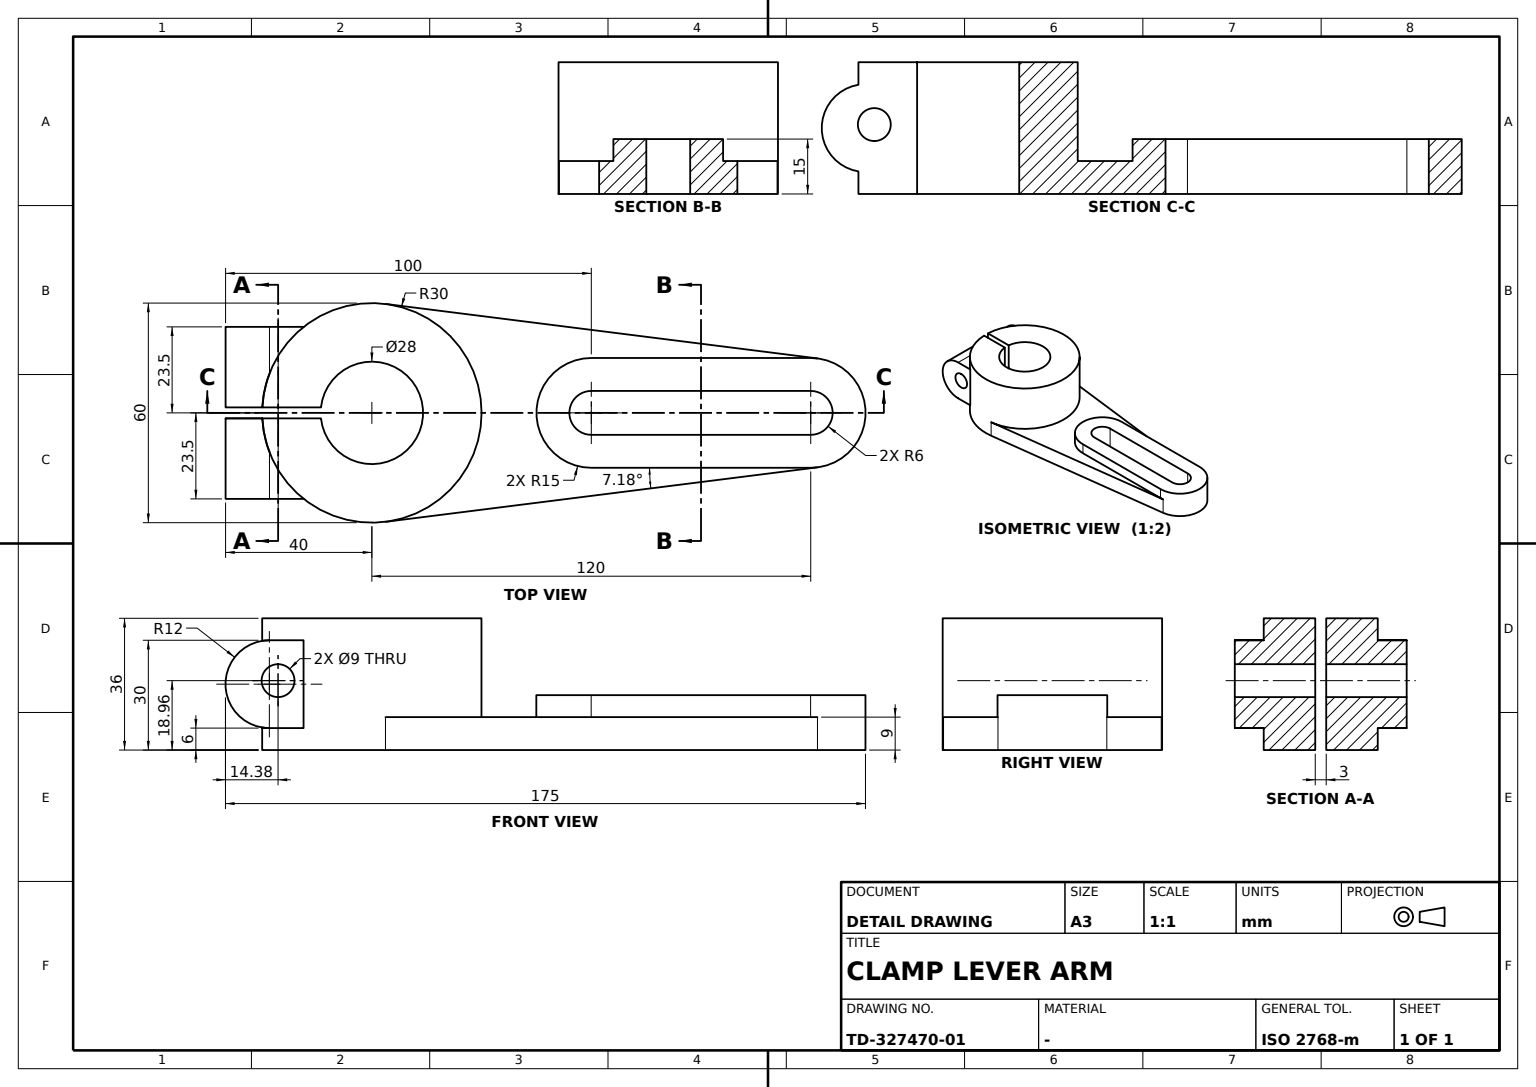
CATIA V5 part; units mm, degrees
sketch "Sketch1" plane through (0, 0, 0) normal (0, 0, 1) x (1, 0, 0)
  circle A0 centre (0, 0) radius 30
  circle A1 centre (0, 0) radius 14
  dimension "radius A1" = 14
  dimension "radius A0" = 30
extrude "Pad1" add sketch "Sketch1" along normal blind 36
sketch "Sketch2" plane through (0, 0, 0) normal (0, 0, 1) x (1, 0, 0)
  line L0 (60, 0) -> (120, 0) construction
  point P0 (60, 0)
  point P1 (120, 0)
  line L1 (60, 15) -> (120, 15)
  line L2 (120, -15) -> (60, -15)
  arc A0 (120, 15) -> (120, -15) centre (120, 0) cw
  arc A1 (60, -15) -> (60, 15) centre (60, 0) cw
  line L3 (60, 0) -> (120, 0) construction
  line L4 (60, 6) -> (120, 6)
  line L5 (120, -6) -> (60, -6)
  arc A2 (120, 6) -> (120, -6) centre (120, 0) cw
  arc A3 (60, -6) -> (60, 6) centre (60, 0) cw
  dimension "distance L0 L1" = 15
  dimension "length L0" = 60
  dimension "distance y axis P1" = 120
  dimension "distance L3 L4" = 6
  constraint coincidence P0 x-axis
  constraint horizontal L0 x-axis
  constraint horizontal L3 x-axis
  constraint tangency A0 L1
  constraint tangency A1 L1
  constraint tangency A0 L2
  constraint tangency A1 L2
  constraint tangency A2 L4
  constraint tangency A3 L4
  constraint tangency A2 L5
  constraint tangency A3 L5
extrude "Pad2" add sketch "Sketch2" along normal blind 15
ref_plane "Plane1" through (0, 0, 3) normal (0, 0, -1) x (1, 0, 0)
sketch "Sketch4" plane through (0, 0, 0) normal (0, 0, -1) x (1, 0, 0)
  circle A0 centre (0, 0) radius 30 construction
  arc A1 (3.75, -29.7647) -> (3.75, 29.7647) centre (0, 0) ccw
  line L0 (120, -15) -> (60, -15)
  point P0 (120, -15)
  arc A2 (120, -15) -> (120, 15) centre (120, 0) ccw construction
  arc A3 (120, -15) -> (121.875, -14.8824) centre (120, 0) ccw
  arc A4 (121.875, 14.8824) -> (120, 15) centre (120, 0) ccw
  point P1 (120, -15)
  point P2 (120, 15)
  line L1 (60, 15) -> (120, 15)
  point P3 (120, 15)
  arc A5 (60, 15) -> (60, -15) centre (60, 0) ccw
  line L2 (3.75, 29.7647) -> (121.875, 14.8824)
  point P4 (3.75, 29.7647)
  point P5 (121.875, 14.8824)
  line L3 (3.75, -29.7647) -> (121.875, -14.8824)
  point P6 (3.75, -29.7647)
  point P7 (121.875, -14.8824)
  constraint tangency L2 A0
  constraint tangency L2 A2
  constraint tangency L3 A0
  constraint tangency L3 A2
  constraint coincidence A0 P4
  constraint coincidence A2 P5
  constraint coincidence A0 P6
  constraint coincidence A2 P7
  constraint coincidence P0 P1
  constraint coincidence P2 P3
extrude "Pad3" add sketch "Sketch4" against normal blind 9
sketch "Sketch5" plane through (0, 0, 0) normal (0, 1, 0) x (-1, 0, 0)
  point P0 (28, 18)
  arc A0 (28, 6) -> (28, 30) centre (28, 18) ccw
  line L0 (28, 30) -> (0, 30)
  point P1 (0, 30)
  line L1 (28, 6) -> (0, 6)
  point P2 (0, 6)
  line L2 (0, 6) -> (0, 30)
  dimension "radius A0" = 12
  dimension "distance P0 x axis" = 18
  dimension "distance y axis P0" = 28
  constraint coincidence P1 y-axis
  constraint coincidence P2 y-axis
  constraint horizontal L0 x-axis
  constraint tangency L1 A0
  constraint vertical L2 y-axis
extrude "Pad4" add sketch "Sketch5" along normal blind 23.5
mirror "Mirror1" about plane through (0, 0, 0) normal (0, 1, 0) of "Pad4"
sketch "Sketch6" plane through (0, 0, 36) normal (0, 0, 1) x (1, 0, 0)
  circle A0 centre (0, 0) radius 14 construction
  arc A1 (-13.9194, -1.5) -> (-13.9194, 1.5) centre (0, 0) ccw
  line L0 (-13.9194, 1.5) -> (-50, 1.5)
  line L1 (-50, 1.5) -> (-50, -1.5)
  line L2 (-50, -1.5) -> (-13.9194, -1.5)
  point P0 (-13.9194, 1.5)
  point P1 (-13.9194, -1.5)
  dimension "distance L0 L2" = 3
  constraint horizontal L0 x-axis
  constraint horizontal L2 x-axis
  constraint vertical L1 y-axis
  constraint symmetry L0 L2 x-axis
  constraint coincidence A0 P0
  constraint coincidence A0 P1
extrude "Pocket1" cut sketch "Sketch6" against normal through all
sketch "Sketch7" plane through (0, -23.5, 0) normal (0, -1, 0) x (1, 0, 0)
  circle A0 centre (-25.6208, 18.9643) radius 4.5
  dimension "radius A0" = 4.5
extrude "Pocket2" cut sketch "Sketch7" against normal through all
sketch "Sketch3" plane through (0, 0, 0) normal (0, 1, 0) x (-1, 0, 0)
